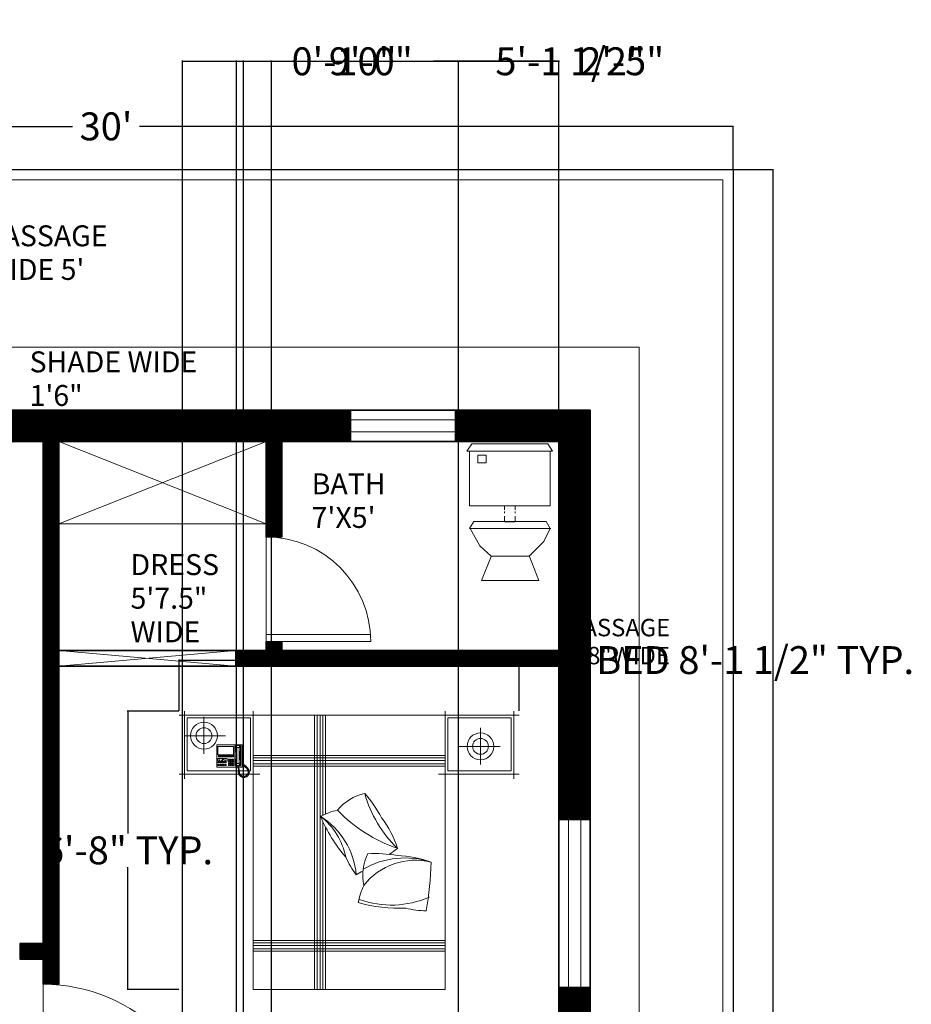
# Model space of a CAD drawing. Units: inches. Extents: x 542 to 1025, y 651 to 1330.
# Tile 4 of 4: x 769 to 1025, y 1048 to 1330. Entities that reach past the tile are written whole.
import ezdxf

# ---------------------------------------------------------------- set-up
doc = ezdxf.new("R2010")
doc.units = ezdxf.units.IN
doc.header["$MEASUREMENT"] = 0
for name, color, linetype, lineweight in [('A-ANNO-DIMS', 2, 'Continuous', 18), ('A-AREA-IDEN', 7, 'Continuous', 18), ('A-DOOR', 3, 'Continuous', 18), ('A-FLOR-CASE', 8, 'Continuous', 18), ('A-FLOR-EXTR', 7, 'Continuous', 18), ('A-FLOR-FIXT', 9, 'Continuous', 18), ('A-GLAZ', 4, 'Continuous', 18), ('A-ROOF', 8, 'Continuous', 18), ('A-WALL', 7, 'Continuous', 35), ('A-WALL-OPEN', 4, 'Continuous', 18), ('A-WALL-PATT', 7, 'Continuous', 13), ('C-PROP', 7, 'Continuous', 25), ('Furniture', 7, 'Continuous', 15)]:
    doc.layers.add(name, color=color, linetype=linetype, lineweight=lineweight)
doc.styles.get("Standard").update_dxf_attribs({"font": 'italic8.shx'})
doc.dimstyles.get("Standard").update_dxf_attribs({"dimtxt": 8, "dimasz": 0.18, "dimexe": 0.18, "dimexo": 0.0625, "dimgap": 0.09, "dimtad": 0, "dimtih": 1, "dimtoh": 1, "dimdec": 4, "dimzin": 0, "dimdsep": 46, "dimlunit": 3, "dimtxsty": 'Standard', "dimcen": 0.09, "dimclrt": 6, "dimadec": 0, "dimazin": 0, "dimtfac": 1, "dimtdec": 4, "dimtofl": 0, "dimtmove": 0, "dimatfit": 3, "dimfxl": 1, "dimtolj": 1, "dimtzin": 0, "dimarcsym": 0})

# ---------------------------------------------------------------- blocks, each defined once
blk = doc.blocks.new('*D3')
at = {"layer": 'A-ANNO-DIMS', "color": 0, "lineweight": -2, "transparency": 16777216}
for p, q in [((614.23, 1287.2), (614.23, 1299.7)), ((614.41, 1299.52), (784.62, 1299.52)), ((974.05, 1299.52), (803.84, 1299.52)), ((974.23, 1287.2), (974.23, 1299.7))]:
    blk.add_line(p, q, dxfattribs=at)
at = {"layer": 'A-ANNO-DIMS', "color": 0, "transparency": 16777216}
for points in [[(614.41, 1299.55), (614.41, 1299.49), (614.23, 1299.52)], [(974.05, 1299.55), (974.05, 1299.49), (974.23, 1299.52)]]:
    blk.add_solid(points, dxfattribs=at)
at = {"layer": 'Defpoints', "color": 0, "transparency": 16777216}
for p in [(974.23, 1299.52), (614.23, 1287.14), (974.23, 1287.14)]:
    blk.add_point(p, dxfattribs=at)
at = {"layer": 'A-ANNO-DIMS', "color": 0, "transparency": 16777216, "insert": (794.23, 1299.52), "char_height": 8, "attachment_point": 5}
blk.add_mtext("\\A1;30'", dxfattribs=at)
blk = doc.blocks.new('*D4')
at = {"layer": 'A-ANNO-DIMS', "color": 0, "lineweight": -2, "transparency": 16777216}
for p, q in [((974.29, 1287.14), (985.84, 1287.14)), ((985.66, 1286.96), (985.66, 991.99)), ((985.66, 687.32), (985.66, 982.29)), ((974.29, 687.14), (985.84, 687.14))]:
    blk.add_line(p, q, dxfattribs=at)
at = {"layer": 'A-ANNO-DIMS', "color": 0, "transparency": 16777216}
for points in [[(985.63, 1286.96), (985.69, 1286.96), (985.66, 1287.14)], [(985.63, 687.32), (985.69, 687.32), (985.66, 687.14)]]:
    blk.add_solid(points, dxfattribs=at)
at = {"layer": 'Defpoints', "color": 0, "transparency": 16777216}
for p in [(974.23, 1287.14), (974.23, 687.14), (985.66, 687.14)]:
    blk.add_point(p, dxfattribs=at)
at = {"layer": 'A-ANNO-DIMS', "color": 0, "transparency": 16777216, "insert": (985.66, 987.14), "char_height": 8, "attachment_point": 5}
blk.add_mtext("\\A1;50'", dxfattribs=at)
blk = doc.blocks.new('BED-DOUBLE-WITH-NIGHTSTANDS')
for p, q in [((1.62, 79.86), (1.62, 60.43)), ((21.28, 79.86), (21.28, 60.43)), ((76.4, 79.86), (76.4, 60.43)), ((96.06, 79.86), (96.06, 60.43)), ((22.78, 78.74), (0.09, 78.74)), ((20.56, 77.92), (2.34, 77.92)), ((2.34, 77.92), (2.34, 62.74)), ((7.16, 67.63), (7.16, 78.19)), ((20.56, 62.74), (20.56, 77.92)), ((21.28, 0), (21.28, 78.74)), ((76.4, 78.74), (21.28, 78.74)), ((38.89, 0), (38.89, 78.74)), ((39.64, 0), (39.64, 78.74)), ((40.53, 0), (40.53, 78.74)), ((41.27, 50.01), (41.27, 78.74)), ((42.02, 50.34), (42.02, 78.74)), ((74.9, 78.74), (97.59, 78.74)), ((76.4, 78.74), (76.4, 0)), ((77.12, 62.74), (77.12, 77.92)), ((77.12, 77.92), (95.34, 77.92)), ((95.34, 77.92), (95.34, 62.74)), ((86.53, 64.55), (86.53, 75.12)), ((1.52, 72.82), (13.32, 72.82)), ((10.94, 70.2), (10.85, 70.11)), ((10.85, 70.11), (10.85, 63.9)), ((10.94, 70.2), (18.05, 70.2)), ((15.62, 69.71), (11.12, 69.71)), ((11.12, 69.71), (11.12, 67.32)), ((15.62, 67.32), (15.62, 69.71)), ((16.03, 69.84), (16.21, 70.07)), ((16.03, 64.4), (16.03, 69.84)), ((16.21, 69.93), (16.16, 69.75)), ((16.16, 69.75), (16.16, 68.54)), ((16.16, 69.75), (16.57, 69.35)), ((16.16, 68.54), (16.25, 68.31)), ((16.21, 70.07), (17.56, 70.07)), ((16.39, 70.02), (16.21, 69.93)), ((16.25, 68.31), (16.39, 68.09)), ((16.39, 70.02), (17.47, 70.02)), ((16.61, 69.44), (16.39, 70.02)), ((16.39, 68.09), (16.43, 67.77)), ((16.57, 69.35), (16.61, 69.44)), ((16.57, 67.32), (16.57, 69.35)), ((17.24, 69.44), (16.61, 69.44)), ((17.24, 69.44), (17.47, 70.02)), ((17.29, 69.35), (17.24, 69.44)), ((17.69, 69.75), (17.29, 69.35)), ((17.29, 67.32), (17.29, 69.35)), ((17.47, 68.09), (17.42, 67.77)), ((17.47, 70.02), (17.65, 69.93)), ((17.6, 68.31), (17.47, 68.09)), ((17.56, 70.07), (17.78, 69.84)), ((17.69, 68.54), (17.6, 68.31)), ((17.65, 69.93), (17.69, 69.75)), ((17.69, 69.75), (17.69, 68.54)), ((17.78, 69.84), (17.78, 64.44)), ((18.05, 70.2), (18.14, 70.11)), ((18.14, 70.11), (18.14, 63.9)), ((92.17, 69.75), (80.38, 69.75)), ((11.12, 67.32), (15.62, 67.32)), ((13.78, 66.29), (11.12, 66.29)), ((11.12, 66.29), (11.12, 65.48)), ((11.12, 65.48), (13.78, 65.48)), ((11.17, 65.25), (11.17, 65.07)), ((11.62, 65.25), (11.17, 65.25)), ((11.17, 65.07), (11.62, 65.07)), ((15.62, 67.23), (11.3, 67.23)), ((11.3, 67.23), (11.3, 66.78)), ((11.3, 66.95), (15.62, 66.95)), ((11.3, 66.78), (15.62, 66.78)), ((11.57, 66.2), (11.57, 66.06)), ((11.71, 66.2), (11.57, 66.2)), ((11.57, 66.06), (11.71, 66.06)), ((11.57, 65.7), (11.57, 65.57)), ((11.71, 65.7), (11.57, 65.7)), ((11.57, 65.57), (11.71, 65.57)), ((11.62, 65.07), (11.62, 65.25)), ((11.66, 67.23), (11.66, 66.78)), ((11.71, 66.06), (11.71, 66.2)), ((11.71, 65.57), (11.71, 65.7)), ((11.8, 65.25), (11.8, 65.07)), ((12.25, 65.25), (11.8, 65.25)), ((11.8, 65.15), (11.9, 65.25)), ((11.8, 65.07), (12.25, 65.07)), ((12.02, 67.23), (12.02, 66.78)), ((12.13, 65.48), (12.94, 66.29)), ((12.25, 65.07), (12.25, 65.25)), ((12.38, 67.23), (12.38, 66.78)), ((12.52, 66.2), (12.38, 66.2)), ((12.38, 66.2), (12.38, 66.06)), ((12.38, 66.06), (12.52, 66.06)), ((12.52, 65.7), (12.38, 65.7)), ((12.38, 65.7), (12.38, 65.57)), ((12.38, 65.57), (12.52, 65.57)), ((12.43, 65.25), (12.43, 65.07)), ((12.88, 65.25), (12.43, 65.25)), ((12.43, 65.07), (12.88, 65.07)), ((12.52, 66.06), (12.52, 66.2)), ((12.52, 65.57), (12.52, 65.7)), ((12.74, 67.23), (12.74, 66.78)), ((12.88, 65.07), (12.88, 65.25)), ((13.51, 65.25), (13.06, 65.25)), ((13.06, 65.25), (13.06, 65.07)), ((13.06, 65.07), (13.51, 65.07)), ((13.1, 67.23), (13.1, 66.78)), ((13.33, 66.2), (13.19, 66.2)), ((13.19, 66.2), (13.19, 66.06)), ((13.19, 66.06), (13.33, 66.06)), ((13.33, 65.7), (13.19, 65.7)), ((13.19, 65.7), (13.19, 65.57)), ((13.19, 65.57), (13.33, 65.57)), ((13.33, 66.06), (13.33, 66.2)), ((13.33, 65.57), (13.33, 65.7)), ((13.43, 66.78), (13.6, 66.95)), ((13.46, 67.23), (13.46, 66.78)), ((13.51, 65.07), (13.51, 65.25)), ((13.78, 65.48), (13.78, 66.29)), ((14.18, 65.79), (14.18, 66.06)), ((14.18, 66.06), (14.54, 66.06)), ((14.54, 65.79), (14.18, 65.79)), ((14.18, 65.3), (14.18, 65.57)), ((14.18, 65.57), (14.54, 65.57)), ((14.54, 65.3), (14.18, 65.3)), ((14.18, 64.76), (14.18, 65.03)), ((14.18, 65.03), (14.54, 65.03)), ((14.54, 66.06), (14.54, 65.79)), ((14.54, 65.57), (14.54, 65.3)), ((14.54, 65.03), (14.54, 64.76)), ((14.72, 66.06), (15.08, 66.06)), ((14.72, 65.79), (14.72, 66.06)), ((15.08, 65.79), (14.72, 65.79)), ((14.72, 65.3), (14.72, 65.57)), ((14.72, 65.57), (15.08, 65.57)), ((15.08, 65.3), (14.72, 65.3)), ((14.72, 65.03), (15.08, 65.03)), ((14.72, 64.76), (14.72, 65.03)), ((15.08, 66.06), (15.08, 65.79)), ((15.08, 65.57), (15.08, 65.3)), ((15.08, 65.03), (15.08, 64.76)), ((15.26, 65.79), (15.26, 66.06)), ((15.26, 66.06), (15.62, 66.06)), ((15.62, 65.79), (15.26, 65.79)), ((15.26, 65.3), (15.26, 65.57)), ((15.26, 65.57), (15.62, 65.57)), ((15.62, 65.3), (15.26, 65.3)), ((15.26, 65.07), (15.62, 65.07)), ((15.26, 64.8), (15.26, 65.07)), ((15.62, 66.78), (15.62, 67.23)), ((15.62, 66.06), (15.62, 65.79)), ((15.62, 65.57), (15.62, 65.3)), ((15.62, 65.07), (15.62, 64.8)), ((16.03, 66.95), (16.43, 66.95)), ((16.16, 65.7), (16.25, 65.93)), ((16.16, 64.49), (16.16, 65.7)), ((16.25, 65.93), (16.39, 66.15)), ((16.39, 66.15), (16.43, 66.47)), ((16.43, 67.77), (16.43, 67.32)), ((16.43, 66.47), (16.43, 67.32)), ((16.57, 67.32), (16.57, 64.89)), ((17.29, 67.32), (17.29, 64.89)), ((17.42, 67.77), (17.42, 67.32)), ((17.42, 66.47), (17.42, 67.32)), ((17.47, 66.15), (17.42, 66.47)), ((17.6, 65.93), (17.47, 66.15)), ((17.69, 65.7), (17.6, 65.93)), ((17.69, 64.49), (17.69, 65.7)), ((76.4, 67.17), (21.28, 67.17)), ((76.4, 66.43), (21.28, 66.43)), ((76.4, 65.68), (21.28, 65.68)), ((2.34, 62.74), (20.56, 62.74)), ((10.85, 63.9), (10.94, 63.81)), ((16.93, 63.81), (10.94, 63.81)), ((11.17, 64.58), (11.62, 64.58)), ((11.17, 64.31), (11.17, 64.58)), ((11.17, 64.52), (11.23, 64.58)), ((11.62, 64.31), (11.17, 64.31)), ((11.62, 64.58), (11.62, 64.31)), ((11.8, 64.58), (12.25, 64.58)), ((11.8, 64.31), (11.8, 64.58)), ((12.25, 64.31), (11.8, 64.31)), ((12.25, 64.58), (12.25, 64.31)), ((12.43, 64.58), (12.88, 64.58)), ((12.43, 64.31), (12.43, 64.58)), ((12.88, 64.31), (12.43, 64.31)), ((12.88, 64.58), (12.88, 64.31)), ((13.06, 64.31), (13.06, 64.58)), ((13.06, 64.58), (13.51, 64.58)), ((13.51, 64.31), (13.06, 64.31)), ((13.51, 64.58), (13.51, 64.31)), ((14.54, 64.76), (14.18, 64.76)), ((14.18, 64.26), (14.18, 64.53)), ((14.18, 64.53), (14.54, 64.53)), ((14.54, 64.26), (14.18, 64.26)), ((14.54, 64.53), (14.54, 64.26)), ((15.08, 64.76), (14.72, 64.76)), ((14.72, 64.26), (14.72, 64.53)), ((14.72, 64.53), (15.08, 64.53)), ((15.08, 64.26), (14.72, 64.26)), ((15.08, 64.53), (15.08, 64.26)), ((15.62, 64.8), (15.26, 64.8)), ((15.26, 64.53), (15.62, 64.53)), ((15.26, 64.26), (15.26, 64.53)), ((15.62, 64.26), (15.26, 64.26)), ((15.62, 64.53), (15.62, 64.26)), ((16.25, 64.17), (16.03, 64.4)), ((16.16, 64.49), (16.57, 64.89)), ((16.21, 64.31), (16.16, 64.49)), ((16.39, 64.22), (16.21, 64.31)), ((16.89, 64.17), (16.25, 64.17)), ((16.61, 64.8), (16.39, 64.22)), ((16.39, 64.22), (16.89, 64.22)), ((16.57, 64.89), (16.61, 64.8)), ((17.24, 64.8), (16.61, 64.8)), ((17.02, 64.35), (16.88, 64.35)), ((16.88, 64.35), (16.89, 63.96)), ((16.89, 63.96), (17, 63.51)), ((17, 63.51), (17.11, 63.08)), ((17.03, 62.69), (17.01, 62.47)), ((17.01, 62.47), (17.27, 62.42)), ((17.04, 63.99), (17.02, 64.35)), ((17.27, 62.42), (17.02, 62.27)), ((17.02, 62.27), (17.03, 62.02)), ((17.03, 64.22), (17.47, 64.22)), ((17.56, 64.17), (17.03, 64.17)), ((17.13, 62.79), (17.03, 62.69)), ((17.11, 63.7), (17.04, 63.99)), ((18.05, 63.81), (17.08, 63.81)), ((17.11, 63.08), (17.1, 62.84)), ((17.1, 62.84), (17.13, 62.79)), ((17.22, 63.27), (17.11, 63.7)), ((17.24, 63.05), (17.22, 63.27)), ((17.29, 64.89), (17.24, 64.8)), ((17.24, 64.8), (17.47, 64.22)), ((17.24, 62.82), (17.24, 63.05)), ((17.4, 62.7), (17.24, 62.82)), ((17.69, 64.49), (17.29, 64.89)), ((17.36, 62.49), (17.4, 62.7)), ((17.41, 61.91), (17.36, 62.49)), ((17.47, 64.22), (17.65, 64.31)), ((17.78, 64.44), (17.56, 64.17)), ((17.65, 64.31), (17.69, 64.49)), ((18.14, 63.9), (18.05, 63.81)), ((18.41, 64.61), (18.14, 64.71)), ((18.14, 64.53), (18.34, 64.48)), ((18.34, 64.48), (18.52, 64.33)), ((18.54, 64.48), (18.41, 64.61)), ((18.52, 64.33), (18.57, 64.27)), ((18.63, 64.4), (18.54, 64.48)), ((18.57, 64.27), (18.67, 64.28)), ((18.67, 64.28), (18.57, 64.18)), ((18.57, 64.18), (18.94, 63.86)), ((18.8, 64.46), (18.63, 64.4)), ((18.88, 64.38), (18.8, 64.46)), ((18.82, 64.25), (18.88, 64.38)), ((18.93, 64.33), (18.82, 64.25)), ((19.05, 64.21), (18.93, 64.33)), ((18.94, 63.86), (19.53, 63.35)), ((18.95, 63.94), (19.05, 64.21)), ((19.2, 64.07), (18.95, 63.94)), ((19.4, 63.87), (19.2, 64.07)), ((19.36, 63.59), (19.4, 63.87)), ((19.56, 63.71), (19.36, 63.59)), ((19.54, 63.33), (19.84, 62.48)), ((19.74, 63.53), (19.56, 63.71)), ((19.67, 63.33), (19.74, 63.53)), ((19.94, 63.36), (19.67, 63.33)), ((19.84, 62.48), (19.71, 61.79)), ((19.76, 62.99), (20.02, 63.09)), ((20.05, 63), (19.76, 62.99)), ((19.92, 62.61), (20.11, 62.79)), ((20.17, 62.61), (19.92, 62.61)), ((19.93, 62.3), (20.21, 62.38)), ((20.17, 62.16), (19.93, 62.3)), ((20.02, 63.09), (19.94, 63.36)), ((20.11, 62.79), (20.05, 63)), ((20.13, 61.98), (20.17, 62.16)), ((20.21, 62.38), (20.17, 62.61)), ((76.4, 64.79), (21.28, 64.79)), ((76.4, 64.04), (21.28, 64.04)), ((95.34, 62.74), (77.12, 62.74)), ((0, 61.81), (23.23, 61.81)), ((17.03, 62.02), (17.33, 62)), ((17.33, 62), (17.07, 61.79)), ((17.07, 61.79), (17.19, 61.59)), ((17.19, 61.59), (17.46, 61.64)), ((17.46, 61.64), (17.34, 61.38)), ((17.34, 61.38), (17.47, 61.22)), ((17.75, 61.48), (17.41, 61.91)), ((17.47, 61.22), (17.68, 61.38)), ((17.68, 61.38), (17.65, 61.13)), ((17.65, 61.13), (17.82, 61.02)), ((18.24, 61.22), (17.75, 61.48)), ((17.82, 61.02), (18.04, 61.2)), ((18.04, 61.2), (18.01, 60.9)), ((18.01, 60.9), (18.2, 60.85)), ((18.2, 60.85), (18.32, 61.09)), ((18.78, 61.18), (18.24, 61.22)), ((18.32, 61.09), (18.43, 60.85)), ((18.43, 60.85), (18.58, 60.83)), ((18.58, 60.83), (18.65, 61.09)), ((18.65, 61.09), (18.75, 60.8)), ((18.75, 60.8), (18.92, 60.85)), ((19.31, 61.4), (18.78, 61.18)), ((18.92, 60.85), (18.93, 61.09)), ((18.93, 61.09), (19.14, 60.91)), ((19.14, 60.91), (19.28, 60.98)), ((19.28, 60.98), (19.26, 61.26)), ((19.26, 61.26), (19.45, 61.02)), ((19.71, 61.79), (19.31, 61.4)), ((19.45, 61.02), (19.59, 61.15)), ((19.59, 61.15), (19.48, 61.39)), ((19.48, 61.39), (19.74, 61.28)), ((19.73, 61.64), (19.99, 61.56)), ((19.86, 61.39), (19.73, 61.64)), ((19.74, 61.95), (19.88, 61.95)), ((19.74, 61.28), (19.86, 61.39)), ((20.07, 61.74), (19.85, 61.99)), ((19.85, 61.99), (20.13, 61.98)), ((19.99, 61.56), (20.07, 61.74)), ((97.68, 61.81), (74.45, 61.81)), ((41.27, 0), (41.27, 48.21)), ((42.02, 0), (42.02, 46.69)), ((76.4, 14.11), (21.28, 14.11)), ((76.4, 13.36), (21.28, 13.36)), ((76.4, 12.62), (21.28, 12.62)), ((76.4, 11.73), (21.28, 11.73)), ((76.4, 10.98), (21.28, 10.98)), ((76.4, 0), (21.28, 0))]:
    blk.add_line(p, q)
for centre, radius in [((7.16, 72.82), 3.85), ((7.16, 72.82), 2.27), ((86.53, 69.75), 3.85), ((86.53, 69.75), 2.27)]:
    blk.add_circle(centre, radius)
for centre, radius, start, end in [((56.35, 42.51), 14.08, 102.4782, 140.4625), ((86.33, 65.31), 34.24, 195.336, 226.4193), ((23.98, 30.71), 38.9, 28.4971, 41.0566), ((50.42, 30.47), 21.57, 103.2034, 117.0362), ((76.26, 80.81), 42.51, 223.6306, 251.4288), ((82.82, 67.66), 45.87, 203.0642, 220.3209), ((28.97, 34.41), 19.21, 10.6986, 52.6864), ((28.71, 30.87), 22.27, 5.3391, 57.6895), ((33.3, 30.75), 31, 18.3527, 36.6851), ((10.36, 109.39), 86.52, 305.2966, 307.2418), ((73.98, 50.3), 28.9, 205.259, 216.9351), ((66.84, 32.82), 14.08, 154.0418, 192.0262), ((64.89, 13.81), 23.96, 71.81, 120.1351), ((67.88, 18.31), 18.8, 76.1849, 142.0017), ((55.96, 0.12), 38.9, 80.0607, 92.6202), ((61.72, 7.45), 31, 69.9163, 88.2487), ((10.36, 109.39), 86.52, 297.9248, 299.3793), ((-14.14, 38.37), 86.52, 349.4884, 358.8054), ((72.58, 20.69), 21.57, 154.767, 168.5998), ((60.98, 51.35), 27.11, 250.2936, 293.6414), ((63.6, 69.18), 45.87, 254.6278, 271.8845), ((71.69, 51.47), 28.9, 256.8226, 268.4988)]:
    blk.add_arc(centre, radius, start, end)
at = {"flags": 9}
for tag in ['XSIZE', 'ZSIZE', 'YSIZE']:
    blk.add_attdef(tag, (57.6, 35.4), '', height=0.0197, rotation=90, dxfattribs=at)
blk = doc.blocks.new('WC-TANK')
for p, q in [((0, 37.14), (1.38, 39.21)), ((0, 37.14), (24.51, 37.14)), ((0.71, 37.14), (0.71, 21.45)), ((1.38, 39.21), (23.19, 39.21)), ((24.51, 37.14), (23.19, 39.21)), ((23.85, 21.45), (23.85, 37.14)), ((3.1, 35.95), (3.1, 33.74)), ((5.47, 35.95), (3.1, 35.95)), ((5.47, 33.74), (5.47, 35.95)), ((3.1, 33.74), (5.47, 33.74)), ((0.71, 21.45), (23.85, 21.45)), ((10.73, 20.35), (10.73, 21.49)), ((10.73, 19.33), (10.73, 19.84)), ((12.28, 21.45), (13.82, 21.45)), ((13.82, 21.45), (13.82, 20.35)), ((13.82, 19.84), (13.82, 19.33)), ((10.73, 16.85), (10.73, 18.48)), ((13.82, 18.48), (13.82, 16.85)), ((0.71, 14.94), (1.99, 16.93)), ((0.71, 14.94), (23.85, 14.94)), ((24.1, 14.94), (0.96, 14.94)), ((0.96, 14.94), (3.7, 9.98)), ((1.99, 16.93), (22.71, 16.93)), ((13.82, 16.85), (10.73, 16.85)), ((22.02, 11.19), (23.85, 14.94)), ((23.85, 14.94), (22.71, 16.93)), ((3.7, 9.98), (6.94, 6.98)), ((17.87, 6.98), (22.02, 11.19)), ((4.14, 0), (6.9, 6.9)), ((17.87, 6.98), (6.94, 6.98)), ((6.94, 6.98), (17.87, 6.98)), ((20.67, 0), (17.91, 6.9)), ((4.14, 0), (20.67, 0)), ((12.4, 0), (4.14, 0))]:
    blk.add_line(p, q)
blk = doc.blocks.new('DOOR-SINGLE-48IN')
for p, q in [((48, 0), (48, 48)), ((0, 0), (48, 0)), ((0.04, 2), (48, 2))]:
    blk.add_line(p, q)
blk.add_arc((48, 0), 48, 90, 180)
blk = doc.blocks.new('DOOR-SINGLE-30IN')
for p, q in [((0, 0), (0, 30)), ((29.93, 2), (0, 2)), ((30, 0), (0, 0))]:
    blk.add_line(p, q)
blk.add_arc((0, 0), 30, 0, 90)
blk = doc.blocks.new('WINDOW-48IN')
for p, q in [((0, 48), (0, 0)), ((9, 48), (0, 48)), ((0, 48), (4.5, 48)), ((2.75, 48), (2.75, 0)), ((6.25, 48), (6.25, 0)), ((9, 0), (9, 48)), ((0, 0), (9, 0))]:
    blk.add_line(p, q)
blk = doc.blocks.new('WINDOW-30IN')
for p, q in [((0, 30), (0, 0)), ((9, 30), (0, 30)), ((0, 30), (4.5, 30)), ((2.75, 30), (2.75, 0)), ((6.25, 30), (6.25, 0)), ((9, 0), (9, 30)), ((0, 0), (9, 0))]:
    blk.add_line(p, q)
blk = doc.blocks.new('*D20')
at = {"layer": 'A-ANNO-DIMS', "color": 0, "lineweight": -2, "transparency": 16777216}
for p, q in [((815.19, 1131.84), (815.19, 1146.61)), ((815.37, 1146.43), (912.68, 1146.43)), ((912.86, 1131.84), (912.86, 1146.61)), ((912.86, 1146.43), (913.04, 1146.43))]:
    blk.add_line(p, q, dxfattribs=at)
at = {"layer": 'A-ANNO-DIMS', "color": 0, "transparency": 16777216}
for points in [[(815.37, 1146.46), (815.37, 1146.4), (815.19, 1146.43)], [(912.68, 1146.46), (912.68, 1146.4), (912.86, 1146.43)]]:
    blk.add_solid(points, dxfattribs=at)
at = {"layer": 'Defpoints', "color": 0, "transparency": 16777216}
for p in [(912.86, 1146.43), (815.19, 1131.78), (912.86, 1131.78)]:
    blk.add_point(p, dxfattribs=at)
at = {"layer": 'A-ANNO-DIMS', "color": 6, "transparency": 16777216, "insert": (980.56, 1146.43), "char_height": 8, "attachment_point": 5}
blk.add_mtext('\\A1;BED 8\'-1 1/2" TYP.', dxfattribs=at)
blk = doc.blocks.new('*D21')
at = {"layer": 'A-ANNO-DIMS', "color": 0, "lineweight": -2, "transparency": 16777216}
for p, q in [((815.12, 1131.78), (800.35, 1131.78)), ((800.53, 1131.6), (800.53, 1096.7)), ((800.53, 1052.1), (800.53, 1087)), ((815.12, 1051.92), (800.35, 1051.92))]:
    blk.add_line(p, q, dxfattribs=at)
at = {"layer": 'A-ANNO-DIMS', "color": 0, "transparency": 16777216}
for points in [[(800.5, 1131.6), (800.56, 1131.6), (800.53, 1131.78)], [(800.5, 1052.1), (800.56, 1052.1), (800.53, 1051.92)]]:
    blk.add_solid(points, dxfattribs=at)
at = {"layer": 'Defpoints', "color": 0, "transparency": 16777216}
for p in [(800.53, 1131.78), (815.19, 1131.78), (815.19, 1051.92)]:
    blk.add_point(p, dxfattribs=at)
at = {"layer": 'A-ANNO-DIMS', "color": 6, "transparency": 16777216, "insert": (800.53, 1091.85), "char_height": 8, "attachment_point": 5}
blk.add_mtext('\\A1;6\'-8" TYP.', dxfattribs=at)
blk = doc.blocks.new('*D26')
at = {"layer": 'A-ANNO-DIMS', "color": 0, "lineweight": -2, "transparency": 16777216}
for p, q in [((816.23, 996.2), (816.23, 1318.37)), ((816.41, 1318.19), (852.23, 1318.19)), ((924.05, 1318.19), (888.22, 1318.19)), ((924.23, 996.2), (924.23, 1318.37))]:
    blk.add_line(p, q, dxfattribs=at)
at = {"layer": 'A-ANNO-DIMS', "color": 0, "transparency": 16777216}
for points in [[(816.41, 1318.22), (816.41, 1318.16), (816.23, 1318.19)], [(924.05, 1318.22), (924.05, 1318.16), (924.23, 1318.19)]]:
    blk.add_solid(points, dxfattribs=at)
at = {"layer": 'Defpoints', "color": 0, "transparency": 16777216}
for p in [(924.23, 1318.19), (816.23, 996.14), (924.23, 996.14)]:
    blk.add_point(p, dxfattribs=at)
at = {"layer": 'A-ANNO-DIMS', "color": 6, "transparency": 16777216, "insert": (870.23, 1318.19), "char_height": 8, "attachment_point": 5}
blk.add_mtext('\\A1;9\'-0"', dxfattribs=at)
blk = doc.blocks.new('*D30')
at = {"layer": 'A-ANNO-DIMS', "color": 0, "lineweight": -2, "transparency": 16777216}
for p, q in [((831.73, 811.7), (831.73, 1318.37)), ((831.91, 1318.19), (841.55, 1318.19)), ((841.73, 811.7), (841.73, 1318.37)), ((841.73, 1318.19), (841.91, 1318.19))]:
    blk.add_line(p, q, dxfattribs=at)
at = {"layer": 'A-ANNO-DIMS', "color": 0, "transparency": 16777216}
for points in [[(831.91, 1318.22), (831.91, 1318.16), (831.73, 1318.19)], [(841.55, 1318.22), (841.55, 1318.16), (841.73, 1318.19)]]:
    blk.add_solid(points, dxfattribs=at)
at = {"layer": 'Defpoints', "color": 0, "transparency": 16777216}
for p in [(841.73, 1318.19), (831.73, 811.64), (841.73, 811.64)]:
    blk.add_point(p, dxfattribs=at)
at = {"layer": 'A-ANNO-DIMS', "color": 6, "transparency": 16777216, "insert": (862.57, 1318.19), "char_height": 8, "attachment_point": 5}
blk.add_mtext('\\A1;0\'-10"', dxfattribs=at)
blk = doc.blocks.new('*D31')
at = {"layer": 'A-ANNO-DIMS', "color": 0, "lineweight": -2, "transparency": 16777216}
for p, q in [((833.7, 932.22), (833.7, 1318.37)), ((833.88, 1318.19), (895.2, 1318.19)), ((895.38, 932.22), (895.38, 1318.37)), ((895.38, 1318.19), (895.56, 1318.19))]:
    blk.add_line(p, q, dxfattribs=at)
at = {"layer": 'A-ANNO-DIMS', "color": 0, "transparency": 16777216}
for points in [[(833.88, 1318.22), (833.88, 1318.16), (833.7, 1318.19)], [(895.2, 1318.22), (895.2, 1318.16), (895.38, 1318.19)]]:
    blk.add_solid(points, dxfattribs=at)
at = {"layer": 'Defpoints', "color": 0, "transparency": 16777216}
for p in [(895.38, 1318.19), (833.7, 932.16), (895.38, 932.16)]:
    blk.add_point(p, dxfattribs=at)
at = {"layer": 'A-ANNO-DIMS', "color": 6, "transparency": 16777216, "insert": (927.46, 1318.19), "char_height": 8, "attachment_point": 5}
blk.add_mtext('\\A1;5\'-1 1/2"', dxfattribs=at)
blk = doc.blocks.new('*D34')
at = {"layer": 'A-ANNO-DIMS', "color": 0, "lineweight": -2, "transparency": 16777216}
for p, q in [((895.38, 964.19), (895.38, 1318.37)), ((895.56, 1318.19), (924.05, 1318.19)), ((924.23, 964.19), (924.23, 1318.37)), ((924.23, 1318.19), (924.41, 1318.19))]:
    blk.add_line(p, q, dxfattribs=at)
at = {"layer": 'A-ANNO-DIMS', "color": 0, "transparency": 16777216}
for points in [[(895.56, 1318.22), (895.56, 1318.16), (895.38, 1318.19)], [(924.05, 1318.22), (924.05, 1318.16), (924.23, 1318.19)]]:
    blk.add_solid(points, dxfattribs=at)
at = {"layer": 'Defpoints', "color": 0, "transparency": 16777216}
for p in [(924.23, 1318.19), (895.38, 964.12), (924.23, 964.12)]:
    blk.add_point(p, dxfattribs=at)
at = {"layer": 'A-ANNO-DIMS', "color": 6, "transparency": 16777216, "insert": (942.4, 1318.19), "char_height": 8, "attachment_point": 5}
blk.add_mtext('\\A1;2\'-5"', dxfattribs=at)

msp = doc.modelspace()

# ---------------------------------------------------------------- hatches: boundary and pattern name
at = {"layer": 'A-WALL-PATT'}
h = msp.add_hatch(dxfattribs=at)
h.set_pattern_fill('ANSI31', color=256)
h.set_pattern_definition([(45, (-552.11989, -271.07657), (-0.088388348, 0.088388348), [])])
h.paths.add_polyline_path([(715.041, 1218.14134), (623.2294, 1218.14134), (623.2294, 1278.14134), (687.2294, 1278.14134), (687.2294, 1287.14134), (614.2294, 1287.14134), (614.2294, 1150.81788), (618.7294, 1150.81788), (623.2294, 1150.81788), (623.2294, 1209.14134), (715.041, 1209.14134)])
h.paths.add_polyline_path([(864.47291, 1213.64134), (864.47291, 1218.14134), (763.041, 1218.14134), (763.041, 1213.64134), (763.041, 1209.14134), (776.2294, 1209.14134), (776.2294, 1065.14134), (769.45548, 1065.14134), (769.45548, 1060.64134), (776.2294, 1060.64134), (776.2294, 1053.42968), (780.7294, 1053.42968), (780.7294, 1144.64134), (780.7294, 1209.14134), (840.2294, 1209.14134), (840.2294, 1181.73273), (844.7294, 1181.73273), (844.7294, 1209.14134), (864.47291, 1209.14134)])
h.paths.add_polyline_path([(933.2294, 1218.14134), (894.47291, 1218.14134), (894.47291, 1209.14134), (924.2294, 1209.14134), (924.2294, 1144.64134), (924.2294, 1100.56821), (928.7294, 1100.56821), (933.2294, 1100.56821)])
h.paths.add_polyline_path([(933.2294, 1052.56821), (924.2294, 1052.56821), (924.2294, 1000.64134), (780.7294, 1000.64134), (780.7294, 1005.42968), (776.2294, 1005.42968), (776.2294, 996.14134), (780.7294, 996.14134), (811.7294, 996.14134), (811.7294, 987.24818), (816.2294, 987.24818), (816.2294, 996.14134), (924.2294, 996.14134), (924.2294, 975.07641), (928.7294, 975.07641), (933.2294, 975.07641)])
h.paths.add_polyline_path([(924.2294, 1149.14134), (844.7294, 1149.14134), (844.7294, 1151.73273), (840.2294, 1151.73273), (840.2294, 1149.14134), (831.41283, 1149.14134), (831.41283, 1144.64134), (924.2294, 1144.64134)])
h.paths.add_polyline_path([(623.2294, 1102.81788), (614.2294, 1102.81788), (614.2294, 1047.96339), (618.7294, 1047.96339), (623.2294, 1047.96339), (623.2294, 1060.64134), (655.18423, 1060.64134), (655.18423, 1065.14134), (623.2294, 1065.14134)])
h.paths.add_polyline_path([(721.45548, 1065.14134), (685.18423, 1065.14134), (685.18423, 1060.64134), (695.2294, 1060.64134), (695.2294, 1000.64134), (623.2294, 1000.64134), (623.2294, 1017.96339), (614.2294, 1017.96339), (614.2294, 996.14134), (666.7294, 996.14134), (666.7294, 976.55402), (671.2294, 976.55402), (675.7294, 976.55402), (675.7294, 996.14134), (699.7294, 996.14134), (699.7294, 1060.64134), (721.45548, 1060.64134)])
h.paths.add_polyline_path([(675.7294, 928.55402), (666.7294, 928.55402), (666.7294, 904.64134), (614.2294, 904.64134), (614.2294, 879.38817), (618.7294, 879.38817), (623.2294, 879.38817), (623.2294, 900.14134), (671.2294, 900.14134), (671.2294, 828.14134), (666.89138, 828.14134), (666.89138, 819.14134), (743.2294, 819.14134), (743.2294, 754.70501), (752.2294, 754.70501), (752.2294, 802.64134), (753.36467, 802.64134), (753.36467, 811.64134), (752.2294, 811.64134), (752.2294, 828.14134), (675.7294, 828.14134)])
h.paths.add_polyline_path([(636.89138, 828.14134), (623.2294, 828.14134), (623.2294, 849.38817), (614.2294, 849.38817), (614.2294, 778.30684), (618.7294, 778.30684), (623.2294, 778.30684), (623.2294, 819.14134), (636.89138, 819.14134)], flags=17)
h.paths.add_polyline_path([(864.47291, 811.64134), (847.39014, 811.64134), (847.39014, 802.64134), (864.47291, 802.64134)], flags=17)
h.paths.add_polyline_path([(817.39014, 811.64134), (807.36467, 811.64134), (807.36467, 802.64134), (817.39014, 802.64134), (817.39014, 807.14134)])
h.paths.add_polyline_path([(933.2294, 927.07641), (924.2294, 927.07641), (924.2294, 900.14134), (816.2294, 900.14134), (816.2294, 951.24818), (811.7294, 951.24818), (811.7294, 895.64134), (928.7294, 895.64134), (928.7294, 811.64134), (894.47291, 811.64134), (894.47291, 802.64134), (933.2294, 802.64134)])
h.paths.add_polyline_path([(752.2294, 706.70501), (743.2294, 706.70501), (743.2294, 696.14134), (712.47774, 696.14134), (712.47774, 691.64134), (712.47774, 687.14134), (752.2294, 687.14134)])
h.paths.add_polyline_path([(664.47774, 696.14134), (623.2294, 696.14134), (623.2294, 730.30684), (614.2294, 730.30684), (614.2294, 687.14134), (664.47774, 687.14134)])
h.paths.add_polyline_path([(925.1985, 1143.73295), (966.26993, 1143.73295), (966.26993, 1152.66152), (925.1985, 1152.66152)], flags=9)
h.paths.add_polyline_path([(925.4366, 1152.0031), (965.31755, 1152.0031), (965.31755, 1159.5031), (925.4366, 1159.5031)], flags=9)

# ---------------------------------------------------------------- linework, layer by layer
at = {"layer": 'A-DOOR'}
for p, q in [((840.2294, 1181.73273), (844.7294, 1181.73273)), ((840.2294, 1151.73273), (844.7294, 1151.73273)), ((769.45548, 1060.64134), (769.45548, 1065.14134)), ((780.7294, 1053.42968), (776.2294, 1053.42968))]:
    msp.add_line(p, q, dxfattribs=at)
at = {"layer": 'A-FLOR-CASE'}
for p, q in [((780.7294, 1185.47854), (840.2294, 1209.14134)), ((840.2294, 1209.14134), (780.7294, 1209.14134)), ((780.7294, 1209.14134), (840.2294, 1185.47854)), ((840.2294, 1185.47854), (780.7294, 1185.47854))]:
    msp.add_line(p, q, dxfattribs=at)
at = {"layer": 'A-FLOR-EXTR'}
for p, q in [((687.2294, 1284.14134), (971.2294, 1284.14134)), ((971.2294, 1284.14134), (971.2294, 802.5643))]:
    msp.add_line(p, q, dxfattribs=at)
at = {"layer": 'A-ROOF'}
for p, q in [((687.2294, 1236.14134), (947.2294, 1236.14134)), ((947.2294, 1236.14134), (947.2294, 802.5643))]:
    msp.add_line(p, q, dxfattribs=at)
at = {"layer": 'A-WALL'}
for p, q in [((623.2294, 1218.14134), (933.2294, 1218.14134)), ((933.2294, 1218.14134), (933.2294, 802.64134)), ((623.2294, 1209.14134), (776.2294, 1209.14134)), ((776.2294, 1065.14134), (776.2294, 1209.14134)), ((780.7294, 1144.64134), (780.7294, 1209.14134)), ((780.7294, 1209.14134), (840.2294, 1209.14134)), ((840.2294, 1209.14134), (840.2294, 1181.73273)), ((844.7294, 1209.14134), (844.7294, 1181.73273)), ((844.7294, 1209.14134), (924.2294, 1209.14134)), ((924.2294, 1209.14134), (924.2294, 1144.64134)), ((840.2294, 1151.73273), (840.2294, 1149.14134)), ((844.7294, 1151.73273), (844.7294, 1149.14134)), ((780.7294, 1149.14134), (840.2294, 1149.14134)), ((844.7294, 1149.14134), (924.2294, 1149.14134)), ((780.7294, 1144.64134), (924.2294, 1144.64134)), ((780.7294, 1053.42968), (780.7294, 1144.64134)), ((924.2294, 1144.64134), (924.2294, 1000.64134)), ((769.45548, 1065.14134), (776.2294, 1065.14134)), ((769.45548, 1060.64134), (776.2294, 1060.64134)), ((776.2294, 1053.42968), (776.2294, 1060.64134))]:
    msp.add_line(p, q, dxfattribs=at)
at = {"layer": 'A-WALL-OPEN'}
for p, q in [((780.7294, 1144.64134), (831.41283, 1149.14134)), ((831.41283, 1144.64134), (780.7294, 1149.14134)), ((831.41283, 1149.14134), (831.41283, 1144.64134)), ((831.41283, 1149.14134), (831.41283, 1144.64134))]:
    msp.add_line(p, q, dxfattribs=at)
at = {"layer": 'C-PROP'}
for p, q in [((614.2294, 1287.14134), (974.2294, 1287.14134)), ((974.2294, 1287.14134), (974.2294, 687.14134))]:
    msp.add_line(p, q, dxfattribs=at)

# ---------------------------------------------------------------- block references
at = {"layer": 'A-DOOR'}
msp.add_blockref('DOOR-SINGLE-30IN', (840.229, 1151.733), dxfattribs=at)
at = {"layer": 'A-DOOR', "extrusion": (0, 0, -1), "zscale": -1}
msp.add_blockref('DOOR-SINGLE-48IN', (-824.2298, 1005.42967), dxfattribs=at)
at = {"layer": 'A-FLOR-FIXT'}
msp.add_blockref('WC-TANK', (897.834, 1169.225), dxfattribs=at)
at = {"layer": 'A-GLAZ', "rotation": 90.00000000000075}
msp.add_blockref('WINDOW-30IN', (894.47308, 1209.14094), dxfattribs=at)
at = {"layer": 'A-GLAZ'}
msp.add_blockref('WINDOW-48IN', (924.229, 1052.568), dxfattribs=at)
at = {"layer": 'Furniture'}
msp.add_blockref('BED-DOUBLE-WITH-NIGHTSTANDS', (815.18562, 1051.92184), dxfattribs=at)

# ---------------------------------------------------------------- texts
at = {"layer": 'A-AREA-IDEN'}
for s, height, p in [('PASSAGE ', 6, (759.344, 1265.12673)), ("WIDE 5'", 6, (759.344, 1255.48826)), ('SHADE WIDE', 6, (772.29559, 1228.97337)), ('1\'6"', 6, (772.29559, 1219.3349)), ('BATH', 6, (853.25959, 1193.98246)), ("7'X5'", 6, (853.25959, 1184.34399)), ('DRESS', 6, (801.27397, 1170.81372)), ('5\'7.5"', 6, (801.27397, 1161.17524)), ('PASSAGE', 5, (926.6866, 1153.2531)), ('WIDE', 6, (801.27397, 1151.53677)), ('2\'8"WIDE', 5, (926.6866, 1145.22104))]:
    msp.add_text(s, height=height, dxfattribs=at).set_placement(p)

# ---------------------------------------------------------------- dimensions: what is measured, and where the dimension line sits
at = {"layer": 'A-ANNO-DIMS'}
for base, p1, p2, override, picture, middle in [((895.38156, 1318.19134), (833.70082, 932.15804), (895.38156, 932.15804), {"dimdec": 1, "dimlfac": 1, "dimrnd": 0, "dimzin": 1, "dimdsep": 46, "dimlunit": 4, "dimfrac": 2}, '*D31', (927.46108, 1318.19134)), ((924.2294, 1318.19134), (816.2294, 996.14134), (924.2294, 996.14134), {"dimdec": 1, "dimlfac": 1, "dimrnd": 0, "dimzin": 1, "dimdsep": 46, "dimlunit": 4, "dimfrac": 2}, '*D26', (870.2294, 1318.19134)), ((841.7294, 1318.19134), (831.7294, 811.64134), (841.7294, 811.64134), {"dimdec": 1, "dimlfac": 1, "dimrnd": 0, "dimzin": 1, "dimdsep": 46, "dimlunit": 4, "dimfrac": 2}, '*D30', (862.57083, 1318.19134)), ((924.2294, 1318.19134), (895.38156, 964.12283), (924.2294, 964.12283), {"dimdec": 1, "dimlfac": 1, "dimrnd": 0, "dimzin": 1, "dimdsep": 46, "dimlunit": 4, "dimfrac": 2}, '*D34', (942.40416, 1318.19134)), ((974.2294, 1299.51674), (614.2294, 1287.14134), (974.2294, 1287.14134), {"dimclrd": 0, "dimclre": 0, "dimclrt": 0}, '*D3', (794.2294, 1299.51674))]:
    dim = msp.add_linear_dim(base=base, p1=p1, p2=p2, dimstyle='Standard', override=override, dxfattribs=at)
    dim.commit()
    dim.dimension.update_dxf_attribs({"geometry": picture, "text_midpoint": middle})
dim = msp.add_linear_dim(base=(985.65631, 687.14134), p1=(974.2294, 1287.14134), p2=(974.2294, 687.14134), angle=90, dimstyle='Standard', override={"dimclrd": 0, "dimclre": 0, "dimclrt": 0}, dxfattribs=at)
dim.commit()
dim.dimension.update_dxf_attribs({"geometry": '*D4', "text_midpoint": (985.65631, 987.14134)})
dim = msp.add_linear_dim(base=(912.86274, 1146.43179), p1=(815.18567, 1131.78023), p2=(912.86274, 1131.78023), text='BED <> TYP.', dimstyle='Standard', override={"dimdec": 1, "dimlfac": 1, "dimrnd": 0, "dimzin": 1, "dimdsep": 46, "dimlunit": 4, "dimfrac": 2}, dxfattribs=at)
dim.commit()
dim.dimension.update_dxf_attribs({"geometry": '*D20', "text_midpoint": (980.56131, 1146.43179)})
dim = msp.add_linear_dim(base=(800.53411, 1131.78023), p1=(815.18567, 1051.92185), p2=(815.18567, 1131.78023), angle=90, text='<> TYP.', dimstyle='Standard', override={"dimdec": 1, "dimlfac": 1, "dimrnd": 0, "dimzin": 1, "dimdsep": 46, "dimlunit": 4, "dimfrac": 2}, dxfattribs=at)
dim.commit()
dim.dimension.update_dxf_attribs({"geometry": '*D21', "text_midpoint": (800.53411, 1091.85104)})

doc.saveas('drawing.dxf')
